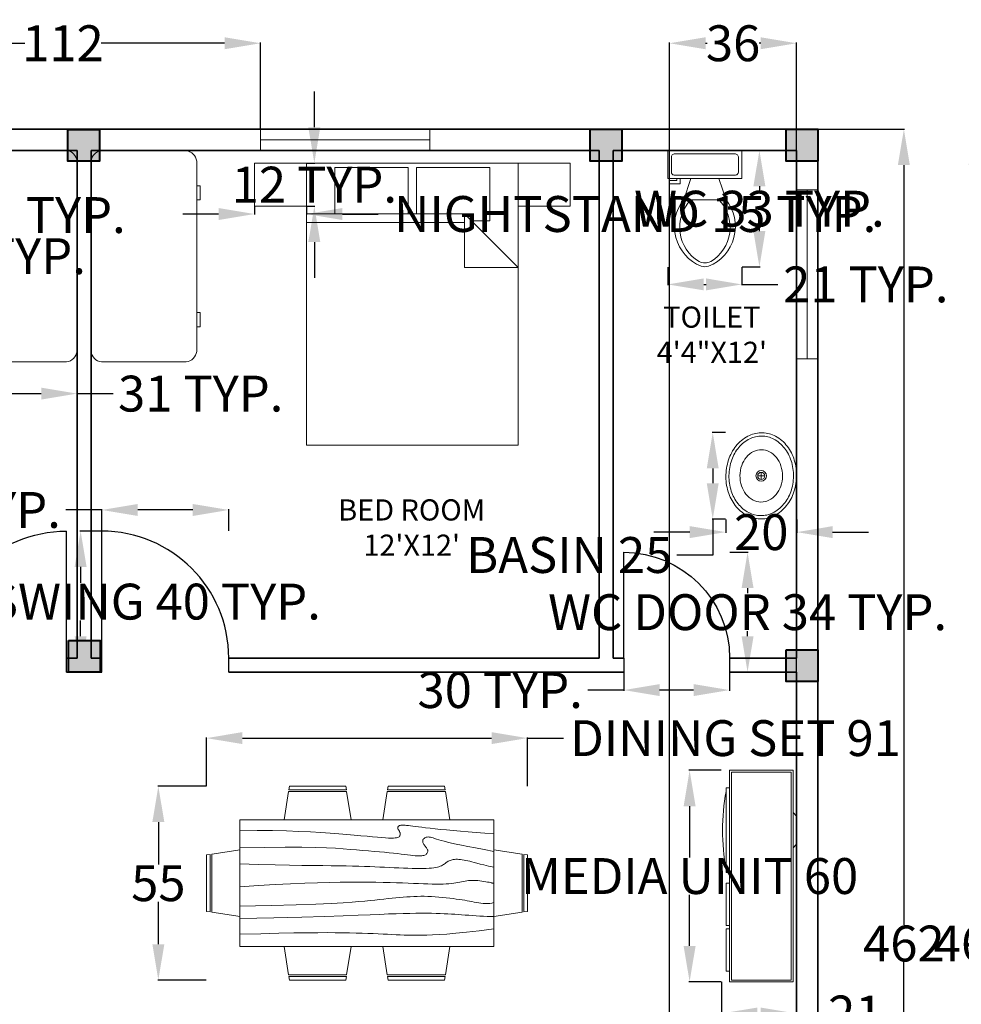
# Model space of a CAD drawing. Units: inches. Extents: x -107 to 647, y -210 to 500.
# Tile 6 of 7: x 183 to 450, y 216 to 495. Entities that reach past the tile are written whole.
import ezdxf

# ---------------------------------------------------------------- set-up
doc = ezdxf.new("R2010")
doc.units = ezdxf.units.IN
doc.header["$MEASUREMENT"] = 0
for name, color, linetype, lineweight in [('A-ANNO-DIMS', 2, 'Continuous', 18), ('A-AREA-IDEN', 7, 'Continuous', 18), ('A-COLS', 7, 'Continuous', 40), ('A-DOOR', 3, 'Continuous', 25), ('A-FLOR-FIXT', 9, 'Continuous', 18), ('A-FURN', 8, 'Continuous', 18), ('A-GLAZ', 4, 'Continuous', 18), ('A-WALL', 7, 'Continuous', 35)]:
    doc.layers.add(name, color=color, linetype=linetype, lineweight=lineweight)
doc.styles.get("Standard").update_dxf_attribs({"font": 'arial.ttf'})
doc.dimstyles.get("Standard").update_dxf_attribs({"dimtxt": 10.18, "dimasz": 10.18, "dimexe": 0.18, "dimexo": 0.0625, "dimgap": 0.09, "dimtad": 0, "dimtih": 1, "dimtoh": 1, "dimdec": 0, "dimzin": 0, "dimdsep": 46, "dimlunit": 3, "dimtxsty": 'Standard', "dimcen": 0.09, "dimadec": 0, "dimazin": 0, "dimtfac": 1, "dimtdec": 0, "dimtofl": 0, "dimtmove": 0, "dimatfit": 3, "dimfxl": 1, "dimtolj": 1, "dimtzin": 0, "dimarcsym": 0})

# ---------------------------------------------------------------- blocks, each defined once
blk = doc.blocks.new('Entertainment Center')
for p, q in [((-4, 0), (-5, -1)), ((4, 0), (-4, 0)), ((5, -1), (4, 0)), ((-17, -19), (-17, -1)), ((-17, -1), (43, -1)), ((-16.5, -18.5), (-16.5, -1.5)), ((-16.5, -1.5), (42.5, -1.5)), ((42.5, -1.5), (42.5, -18.5)), ((43, -1), (43, -19)), ((43, -19), (-17, -19)), ((42.5, -18.5), (-16.5, -18.5)), ((-12, -20), (-12, -19)), ((12, -19), (12, -20)), ((15, -20), (15, -19)), ((27, -19), (27, -20)), ((28, -20), (28, -19)), ((40, -19), (40, -20)), ((12, -20), (-12, -20)), ((27, -20), (15, -20)), ((40, -20), (28, -20))]:
    blk.add_line(p, q)
blk.add_arc((0, 40), 61, 259.6111, 280.3889)
blk = doc.blocks.new('Bed - Queen')
for p, q in [((0, -80.00003), (0, 0)), ((0, 0), (59.99999, 0)), ((59.99999, 0), (59.99999, -80.00003)), ((7.99999, -1.2), (28.79998, -1.2)), ((7.99999, -14.4), (7.99999, -1.2)), ((28.79998, -1.2), (28.79998, -14.4)), ((31.19999, -1.2), (51.99999, -1.2)), ((31.19999, -14.4), (31.19999, -1.2)), ((51.99999, -1.2), (51.99999, -16.4)), ((0, -14.4), (44.8, -14.4)), ((59.99999, -29.6), (44.8, -14.4)), ((44.8, -14.4), (44.8, -29.6)), ((51.99999, -16.4), (46.79936, -16.4)), ((44.8, -16.8), (0, -16.8)), ((44.8, -29.6), (59.99999, -29.6)), ((59.99999, -80.00003), (0, -80.00003))]:
    blk.add_line(p, q)
blk = doc.blocks.new('Desk - 30 x 60 in.')
for p, q in [((-26.999995, 0), (26.999995, 0)), ((-29.999995, -27), (-29.999995, -3)), ((29.999995, -3), (29.999995, -27)), ((26.999995, -30), (-26.999995, -30)), ((-20.000005, -30), (-20.000005, -31)), ((-16.000005, -31), (-16.000005, -30)), ((15.999995, -31), (15.999995, -30)), ((19.999995, -30), (19.999995, -31)), ((-20.000005, -31), (-16.000005, -31)), ((19.999995, -31), (15.999995, -31))]:
    blk.add_line(p, q)
for centre, start, end in [((-26.499995, -3.5), 98.1301, 171.8699), ((26.499995, -3.5), 8.130102, 81.8699), ((-26.499995, -26.5), 188.1301, 261.8699), ((26.499995, -26.5), 278.1301, 351.8699)]:
    blk.add_arc(centre, 3.535534, start, end)
blk = doc.blocks.new('Dining Set - 36 x 72 in.')
for p, q in [((-22.2343, 26.00059), (-23.4847, 17.99762)), ((-22.2304, 26), (-5.7608, 26)), ((-22, 27.5), (-22.1562, 26.50042)), ((-5.8416, 26.5), (-22.1534, 26.5)), ((-22, 27.5), (-6, 27.5)), ((-5.8437, 26.49966), (-6, 27.5)), ((-4.5152, 17.99762), (-5.7655, 25.99926)), ((5.7657, 26.00059), (4.5153, 17.99762)), ((5.7696, 26), (22.2392, 26)), ((6, 27.5), (5.8438, 26.50042)), ((22.1584, 26.5), (5.8466, 26.5)), ((6, 27.5), (22, 27.5)), ((22.1563, 26.49966), (22, 27.5)), ((23.4848, 17.99762), (22.2345, 25.99926)), ((36, 18), (-36, 18)), ((-36, 18), (-36, -18)), ((36, -18), (36, 18)), ((-44.0006, 8.23428), (-35.9976, 9.48474)), ((44.0006, 8.23428), (35.9976, 9.48474)), ((-45.5, 8), (-44.5004, 8.15617)), ((-45.5, 8), (-45.5, -8)), ((-44.5, -8.15843), (-44.5, 8.15338)), ((-44, 8.23041), (-44, -8.23915)), ((44, 8.23041), (44, -8.23915)), ((44.5, -8.15843), (44.5, 8.15338)), ((45.5, 8), (44.5005, 8.15617)), ((45.5, 8), (45.5, -8)), ((-44.4997, -8.15631), (-45.5, -8)), ((-35.9976, -9.48476), (-43.9993, -8.2345)), ((35.9976, -9.48476), (43.9993, -8.2345)), ((44.4997, -8.15631), (45.5, -8)), ((-36, -18), (36, -18)), ((-22.2343, -26.0006), (-23.4847, -17.99762)), ((-4.5152, -17.99762), (-5.7655, -25.99928)), ((5.7657, -26.0006), (4.5153, -17.99762)), ((23.4848, -17.99762), (22.2345, -25.99928)), ((-22.2304, -26), (-5.7608, -26)), ((-22, -27.5), (-22.1562, -26.50044)), ((-5.8416, -26.5), (-22.1534, -26.5)), ((-22, -27.5), (-6, -27.5)), ((-5.8437, -26.49967), (-6, -27.5)), ((5.7696, -26), (22.2392, -26)), ((6, -27.5), (5.8438, -26.50044)), ((22.1584, -26.5), (5.8466, -26.5)), ((6, -27.5), (22, -27.5)), ((22.1563, -26.49967), (22, -27.5))]:
    blk.add_line(p, q)
for points in [[(-36, 15), (-31.1772, 14.97754), (-26.8079, 14.91406), (-22.8538, 14.81543), (-19.276, 14.6875), (-16.0362, 14.53613), (-13.0957, 14.36718), (-10.4159, 14.18652), (-7.9583, 14), (-5.6904, 13.81315), (-3.6035, 13.63021), (-1.6954, 13.45508), (0.0365, 13.29166), (1.5945, 13.14388), (2.9811, 13.01562), (4.1988, 12.9108), (5.25, 12.83333), (6.1393, 12.78613), (6.8802, 12.76823), (7.4883, 12.77767), (7.9792, 12.8125), (8.3685, 12.87077), (8.6719, 12.95052), (8.9049, 13.0498), (9.0833, 13.16666), (9.2205, 13.29899), (9.3216, 13.44401), (9.3895, 13.59879), (9.4271, 13.76041), (9.4373, 13.92594), (9.4232, 14.09245), (9.3875, 14.257), (9.3333, 14.41666), (9.2638, 14.56917), (9.1836, 14.71484), (9.0975, 14.85465), (9.0104, 14.98958), (8.9272, 15.1206), (8.8529, 15.2487), (8.7922, 15.37483), (8.75, 15.5), (8.7305, 15.62467), (8.7344, 15.74739), (8.7617, 15.86621), (8.8125, 15.97916), (8.8867, 16.08431), (8.9844, 16.17968), (9.1055, 16.26334), (9.25, 16.33333), (9.4189, 16.38802), (9.6172, 16.42708), (9.8506, 16.45052), (10.125, 16.45833), (10.4463, 16.45052), (10.8203, 16.42708), (11.2529, 16.38802), (11.75, 16.33333), (12.3184, 16.26318), (12.9694, 16.17838), (13.7151, 16.07991), (14.5677, 15.96875), (15.5395, 15.84586), (16.6426, 15.71224), (17.8893, 15.56884), (19.2917, 15.41666), (20.859, 15.25667), (22.5879, 15.08984), (24.4721, 14.91715), (26.5052, 14.73958), (28.6809, 14.5581), (30.9929, 14.3737), (33.4347, 14.18733), (36, 14)], [(-36, 10), (-28.9766, 10.14274), (-23.1725, 10.20442), (-18.4241, 10.19775), (-14.5677, 10.13541), (-11.4399, 10.03011), (-8.877, 9.89453), (-6.7154, 9.74137), (-4.7917, 9.58333), (-2.9698, 9.43082), (-1.2246, 9.28515), (0.4415, 9.14534), (2.026, 9.01041), (3.5266, 8.87939), (4.9408, 8.7513), (6.266, 8.62516), (7.5, 8.5), (8.6411, 8.37549), (9.6914, 8.2539), (10.6538, 8.13818), (11.5312, 8.03125), (12.3267, 7.93603), (13.043, 7.85547), (13.6831, 7.79248), (14.25, 7.75), (14.7471, 7.7303), (15.1797, 7.73307), (15.5537, 7.75732), (15.875, 7.80208), (16.1494, 7.86637), (16.3828, 7.94922), (16.5811, 8.04964), (16.75, 8.16666), (16.8944, 8.29915), (17.0143, 8.44531), (17.1089, 8.60319), (17.1771, 8.77083), (17.218, 8.94629), (17.2305, 9.1276), (17.2137, 9.31282), (17.1667, 9.5), (17.0895, 9.6875), (16.987, 9.875), (16.8649, 10.0625), (16.7292, 10.25), (16.5856, 10.4375), (16.4401, 10.625), (16.2985, 10.8125), (16.1667, 11), (16.05, 11.18733), (15.9518, 11.3737), (15.8752, 11.5581), (15.8229, 11.73958), (15.798, 11.91715), (15.8034, 12.08984), (15.842, 12.25667), (15.9167, 12.41666), (16.0295, 12.56836), (16.1784, 12.70833), (16.3605, 12.83268), (16.5729, 12.9375), (16.8127, 13.01888), (17.0768, 13.07291), (17.3625, 13.0957), (17.6667, 13.08333), (17.9894, 13.03312), (18.3418, 12.94726), (18.7382, 12.82918), (19.1927, 12.68229), (19.7195, 12.51001), (20.3327, 12.31575), (21.0465, 12.10294), (21.875, 11.875), (22.8357, 11.63354), (23.959, 11.37304), (25.2786, 11.08618), (26.8282, 10.76562), (28.6414, 10.40405), (30.752, 9.99414), (33.1936, 9.52856), (36, 9)], [(-36, 5.5), (-30.7157, 5.3348), (-26.069, 5.20963), (-21.9946, 5.11767), (-18.4271, 5.05208), (-15.3009, 5.00602), (-12.5508, 4.97265), (-10.1112, 4.94515), (-7.9167, 4.91666), (-5.909, 4.88167), (-4.0586, 4.83984), (-2.3429, 4.79215), (-0.7396, 4.73958), (0.7739, 4.6831), (2.22, 4.6237), (3.6213, 4.56233), (5, 4.5), (6.373, 4.43782), (7.7344, 4.3776), (9.0723, 4.32129), (10.375, 4.27083), (11.6309, 4.22819), (12.8281, 4.19531), (13.9551, 4.17415), (15, 4.16666), (15.954, 4.17448), (16.819, 4.19791), (17.6001, 4.23698), (18.3021, 4.29166), (18.9299, 4.36198), (19.4883, 4.44791), (19.9823, 4.54948), (20.4167, 4.66666), (20.7969, 4.79899), (21.1302, 4.94401), (21.4245, 5.09879), (21.6875, 5.26041), (21.9271, 5.42594), (22.1511, 5.59245), (22.3672, 5.757), (22.5834, 5.91666), (22.8065, 6.06868), (23.0404, 6.21093), (23.2879, 6.34147), (23.5521, 6.45833), (23.8358, 6.55957), (24.142, 6.64323), (24.4735, 6.70735), (24.8334, 6.75), (25.2235, 6.76969), (25.642, 6.76692), (26.0858, 6.74267), (26.5521, 6.69791), (27.0379, 6.63362), (27.5404, 6.55078), (28.0565, 6.45036), (28.5834, 6.33333), (29.1242, 6.19987), (29.7071, 6.04687), (30.3661, 5.87044), (31.1354, 5.66666), (32.0493, 5.43164), (33.142, 5.16146), (34.4475, 4.85221), (36, 4.5)], [(-36, -1), (-30.7915, -0.6591), (-26.0195, -0.38216), (-21.6519, -0.16284), (-17.6563, 0.00521), (-14.0005, 0.12833), (-10.6523, 0.21289), (-7.5796, 0.26522), (-4.75, 0.29166), (-2.134, 0.29793), (0.2878, 0.28711), (2.5317, 0.26163), (4.6146, 0.22396), (6.5529, 0.17651), (8.3633, 0.12174), (10.0623, 0.06209), (11.6667, 0), (13.1899, -0.06201), (14.6341, -0.1211), (15.9982, -0.17432), (17.2813, -0.21875), (18.4823, -0.25147), (19.6003, -0.26953), (20.6343, -0.27002), (21.5834, -0.25), (22.4481, -0.20768), (23.2357, -0.14584), (23.9549, -0.06836), (24.6146, 0.02083), (25.2235, 0.11784), (25.7904, 0.21875), (26.3241, 0.31966), (26.8334, 0.41666), (27.3265, 0.50618), (27.8099, 0.58593), (28.2894, 0.65397), (28.7709, 0.70833), (29.2601, 0.74707), (29.763, 0.76823), (30.2855, 0.76985), (30.8334, 0.75), (31.4088, 0.70784), (31.9994, 0.64713), (32.589, 0.57275), (33.1615, 0.48958), (33.7008, 0.4025), (34.1908, 0.3164), (34.6153, 0.23616), (34.9584, 0.16666), (35.2099, 0.11165), (35.3848, 0.07031), (35.504, 0.04069), (35.5886, 0.02083), (35.6594, 0.00879), (35.7377, 0.0026), (35.8442, 0.00032), (36, 0)], [(-36, -6.5), (-27.1843, -6.31267), (-20.084, -6.1263), (-14.469, -5.9419), (-10.1094, -5.76042), (-6.7752, -5.58285), (-4.2363, -5.41016), (-2.2629, -5.24333), (-0.625, -5.08334), (0.8708, -4.93099), (2.2715, -4.78646), (3.5872, -4.64974), (4.8281, -4.52084), (6.0046, -4.39974), (7.127, -4.28646), (8.2053, -4.18099), (9.25, -4.08334), (10.2705, -3.99382), (11.2734, -3.91407), (12.2647, -3.84603), (13.25, -3.79167), (14.2354, -3.75293), (15.2266, -3.73177), (16.2295, -3.73015), (17.25, -3.75), (18.2912, -3.79248), (19.3451, -3.85547), (20.4009, -3.93604), (21.4479, -4.03125), (22.4754, -4.13819), (23.4727, -4.25391), (24.4289, -4.37549), (25.3334, -4.5), (26.1785, -4.62492), (26.9694, -4.74935), (27.7145, -4.87281), (28.4219, -4.99479), (29.1, -5.11483), (29.7572, -5.23242), (30.4016, -5.34709), (31.0417, -5.45834), (31.6837, -5.56437), (32.3262, -5.65821), (32.9658, -5.73153), (33.599, -5.77604), (34.2224, -5.78345), (34.8327, -5.74545), (35.4264, -5.65373), (36, -5.5)], [(-36, -10), (-26.4022, -9.81299), (-18.4675, -9.62891), (-11.9839, -9.45069), (-6.7396, -9.28125), (-2.5226, -9.12354), (0.8789, -8.98047), (3.6769, -8.85498), (6.0833, -8.75), (8.2767, -8.66765), (10.3021, -8.60677), (12.1712, -8.56543), (13.8958, -8.54167), (15.4876, -8.53353), (16.9583, -8.53907), (18.3197, -8.55632), (19.5834, -8.58334), (20.7616, -8.61841), (21.8685, -8.66081), (22.9188, -8.71004), (23.9271, -8.76563), (24.9081, -8.82707), (25.8763, -8.89388), (26.8465, -8.96558), (27.8334, -9.04167), (28.8474, -9.12118), (29.8828, -9.20117), (30.93, -9.27824), (31.9792, -9.34896), (33.0205, -9.40991), (34.0443, -9.45768), (35.0407, -9.48885), (36, -9.5)], [(-36, -14.5), (-30.0881, -14.33513), (-25.0332, -14.21224), (-20.7312, -14.12647), (-17.0781, -14.07292), (-13.97, -14.04671), (-11.3027, -14.04297), (-8.9724, -14.05681), (-6.875, -14.08334), (-4.9224, -14.11833), (-3.0905, -14.16016), (-1.3709, -14.20785), (0.2448, -14.26042), (1.7647, -14.3169), (3.1973, -14.3763), (4.5507, -14.43767), (5.8333, -14.5), (7.0554, -14.5621), (8.235, -14.62175), (9.3922, -14.67652), (10.5469, -14.72396), (11.7192, -14.76164), (12.929, -14.78711), (14.1965, -14.79794), (15.5417, -14.79167), (16.9933, -14.76424), (18.6152, -14.70508), (20.4804, -14.60197), (22.6615, -14.44271), (25.2312, -14.21509), (28.2624, -13.9069), (31.8277, -13.50594), (36, -13)]]:
    blk.add_lwpolyline(points)
blk = doc.blocks.new('Sink - Oval top')
for p, q in [((-1, 0), (1, 0)), ((0, 1), (0, -1))]:
    blk.add_line(p, q)
for points in [[(-12.23, 0.39, 0.117634), (-11.46, -3.36, 0.104469), (-8.88, -6.8, 0.090016), (-5.08, -9.07, 0.08192), (-0.32, -10.02, 0.08192), (4.49, -9.38, 0.090016), (8.42, -7.36, 0.104469), (11.22, -4.09, 0.117634), (12.23, -0.39, 0.117634), (11.46, 3.36, 0.104469), (8.88, 6.8, 0.090016), (5.08, 9.07, 0.08192), (0.32, 10.02, 0.08192), (-4.49, 9.38, 0.090016), (-8.42, 7.36, 0.104469), (-11.22, 4.09, 0.117634)], [(-11.29, 0.16, 0.118622), (-10.52, -3.25, 0.104678), (-8.07, -6.36, 0.089562), (-4.54, -8.37, 0.081185), (-0.13, -9.15, 0.081185), (4.3, -8.49, 0.089562), (7.89, -6.58, 0.104678), (10.42, -3.55, 0.118622), (11.29, -0.16, 0.118622), (10.52, 3.25, 0.104678), (8.07, 6.36, 0.089562), (4.54, 8.37, 0.081185), (0.13, 9.15, 0.081185), (-4.3, 8.49, 0.089562), (-7.89, 6.58, 0.104678), (-10.42, 3.55, 0.118622)], [(-7.42, 0.08, 0.118283), (-6.91, -2.17, 0.104607), (-5.29, -4.21, 0.089718), (-2.97, -5.53, 0.081436), (-0.07, -6.04, 0.081436), (2.84, -5.59, 0.089718), (5.2, -4.33, 0.104607), (6.86, -2.32, 0.118283), (7.42, -0.08, 0.118283), (6.91, 2.17, 0.104607), (5.29, 4.21, 0.089718), (2.97, 5.53, 0.081436), (0.07, 6.04, 0.081436), (-2.84, 5.59, 0.089718), (-5.2, 4.33, 0.104607), (-6.86, 2.32, 0.118283)]]:
    blk.add_lwpolyline(points, format="xyb", close=True)
for radius in [1.5, 1]:
    blk.add_circle((0, 0), radius)
blk = doc.blocks.new('Toilet - top')
for p, q in [((9.5, -6), (9.5, -2)), ((-8, -8.5), (-8, -8)), ((-7, -8), (-7, -9.5)), ((-4, -8), (-6, -14)), ((4, -8), (6, -14)), ((-10, -8.5), (-8, -8.5)), ((-10, -9.5), (-10, -8.5)), ((-7, -9.5), (-10, -9.5)), ((4, -14), (-4, -14))]:
    blk.add_line(p, q)
blk.add_lwpolyline([(10.5, -8), (10.5, 0), (-10.5, 0), (-10.5, -8)], close=True)
for points in [[(-9.5, -2), (-9.5, -6)], [(8.5, -1), (-8.5, -1)], [(-8.5, -7), (8.5, -7)]]:
    blk.add_lwpolyline(points)
for centre, radius, start, end in [((-8.62, -1.88), 0.884, 81.8699, 188.1301), ((8.62, -1.88), 0.884, 351.8699, 98.1301), ((-8.62, -6.12), 0.884, 171.8699, 278.1301), ((8.62, -6.12), 0.884, 261.8699, 8.1301), ((3.52, -21.58), 12.17, 141.4691, 247.9714), ((4.2, -21.82), 11.33, 136.3677, 238.9468), ((-3.52, -21.58), 12.17, 292.0284, 38.5307), ((-4.2, -21.82), 11.33, 301.053, 43.6321), ((0, -27.88), 4, 245.7318, 294.2682), ((0, -29), 4, 254.8605, 285.1395)]:
    blk.add_arc(centre, radius, start, end)
blk = doc.blocks.new('DOOR-SWING-36IN')
for p, q in [((-36, 4), (-36, 0)), ((0, 4), (0, 0)), ((0, 0), (0, -36))]:
    blk.add_line(p, q)
blk.add_arc((0, 0), 36, 180, 270)
blk = doc.blocks.new('DOOR-SWING-30IN')
for p, q in [((0, 0), (4, 0)), ((0, 0), (-30, 0)), ((0, -30), (4, -30))]:
    blk.add_line(p, q)
blk.add_arc((0, 0), 30, 180, 270)
blk = doc.blocks.new('WINDOW-48IN')
for p, q in [((0, 6), (0, 0)), ((48, 6), (48, 0)), ((0, 3), (48, 3))]:
    blk.add_line(p, q)
blk = doc.blocks.new('NIGHTSTAND-15IN')
blk.add_lwpolyline([(14.75, 12.23), (0, 12.23), (0, 0), (14.75, 0)], close=True)
blk = doc.blocks.new('COLUMN-9X9IN')
blk.add_lwpolyline([(0, 9), (9, 9), (9, 0), (0, 0)], close=True)
blk.add_solid([(0, 9), (0, 0), (9, 9), (9, 0)])
blk = doc.blocks.new('*D30')
at = {"layer": 'A-ANNO-DIMS', "color": 0, "lineweight": -2, "transparency": 16777216}
for p, q in [((206.02, 350.33), (199.9, 350.33)), ((200.08, 340.15), (200.08, 335.68)), ((200.08, 320.51), (200.08, 324.97)), ((206.02, 310.33), (199.9, 310.33))]:
    blk.add_line(p, q, dxfattribs=at)
at = {"layer": 'A-ANNO-DIMS', "color": 0, "transparency": 16777216}
for points in [[(198.39, 340.15), (201.78, 340.15), (200.08, 350.33)], [(198.39, 320.51), (201.78, 320.51), (200.08, 310.33)]]:
    blk.add_solid(points, dxfattribs=at)
at = {"layer": 'Defpoints', "color": 0, "transparency": 16777216}
for p in [(206.08, 350.33), (200.08, 310.33), (206.08, 310.33)]:
    blk.add_point(p, dxfattribs=at)
at = {"layer": 'A-ANNO-DIMS', "color": 0, "transparency": 16777216, "insert": (200.08, 330.33), "char_height": 10.18, "attachment_point": 5}
blk.add_mtext('\\A1;DOOR SWING 40 TYP.', dxfattribs=at)
blk = doc.blocks.new('*D31')
at = {"layer": 'A-ANNO-DIMS', "color": 0, "lineweight": -2, "transparency": 16777216}
for p, q in [((206.08, 356.33), (195.9, 356.33)), ((206.08, 350.39), (206.08, 356.51)), ((231.9, 356.33), (216.26, 356.33)), ((242.08, 350.39), (242.08, 356.51))]:
    blk.add_line(p, q, dxfattribs=at)
at = {"layer": 'A-ANNO-DIMS', "color": 0, "transparency": 16777216}
for points in [[(216.26, 358.02), (216.26, 354.63), (206.08, 356.33)], [(231.9, 358.02), (231.9, 354.63), (242.08, 356.33)]]:
    blk.add_solid(points, dxfattribs=at)
at = {"layer": 'Defpoints', "color": 0, "transparency": 16777216}
for p in [(206.08, 356.33), (206.08, 350.33), (242.08, 350.33)]:
    blk.add_point(p, dxfattribs=at)
at = {"layer": 'A-ANNO-DIMS', "color": 0, "transparency": 16777216, "insert": (171.04, 356.33), "char_height": 10.18, "attachment_point": 5}
blk.add_mtext('\\A1;36 TYP.', dxfattribs=at)
blk = doc.blocks.new('*D32')
at = {"layer": 'A-ANNO-DIMS', "color": 0, "lineweight": -2, "transparency": 16777216}
for p, q in [((384.14, 344.33), (389.36, 344.33)), ((389.18, 334.15), (389.18, 332.69)), ((389.18, 320.51), (389.18, 321.96)), ((384.14, 310.33), (389.36, 310.33))]:
    blk.add_line(p, q, dxfattribs=at)
at = {"layer": 'A-ANNO-DIMS', "color": 0, "transparency": 16777216}
for points in [[(387.49, 334.15), (390.88, 334.15), (389.18, 344.33)], [(387.49, 320.51), (390.88, 320.51), (389.18, 310.33)]]:
    blk.add_solid(points, dxfattribs=at)
at = {"layer": 'Defpoints', "color": 0, "transparency": 16777216}
for p in [(384.08, 344.33), (384.08, 310.33), (389.18, 310.33)]:
    blk.add_point(p, dxfattribs=at)
at = {"layer": 'A-ANNO-DIMS', "color": 0, "transparency": 16777216, "insert": (389.18, 327.33), "char_height": 10.18, "attachment_point": 5}
blk.add_mtext('\\A1;WC DOOR 34 TYP.', dxfattribs=at)
blk = doc.blocks.new('*D33')
at = {"layer": 'A-ANNO-DIMS', "color": 0, "lineweight": -2, "transparency": 16777216}
for p, q in [((354.08, 310.26), (354.08, 305.05)), ((384.08, 310.26), (384.08, 305.05)), ((354.08, 305.23), (343.9, 305.23)), ((373.9, 305.23), (364.26, 305.23))]:
    blk.add_line(p, q, dxfattribs=at)
at = {"layer": 'A-ANNO-DIMS', "color": 0, "transparency": 16777216}
for points in [[(364.26, 306.92), (364.26, 303.53), (354.08, 305.23)], [(373.9, 306.92), (373.9, 303.53), (384.08, 305.23)]]:
    blk.add_solid(points, dxfattribs=at)
at = {"layer": 'Defpoints', "color": 0, "transparency": 16777216}
for p in [(354.08, 310.33), (384.08, 310.33), (354.08, 305.23)]:
    blk.add_point(p, dxfattribs=at)
at = {"layer": 'A-ANNO-DIMS', "color": 0, "transparency": 16777216, "insert": (319.04, 305.23), "char_height": 10.18, "attachment_point": 5}
blk.add_mtext('\\A1;30 TYP.', dxfattribs=at)
blk = doc.blocks.new('*D38')
at = {"layer": 'A-ANNO-DIMS', "color": 0, "lineweight": -2, "transparency": 16777216}
for p, q in [((382.93, 378.28), (379.13, 378.28)), ((379.31, 368.1), (379.31, 363.91)), ((382.93, 353.73), (379.13, 353.73)), ((379.31, 353.73), (379.31, 343.55)), ((379.31, 343.55), (369.13, 343.55))]:
    blk.add_line(p, q, dxfattribs=at)
at = {"layer": 'A-ANNO-DIMS', "color": 0, "transparency": 16777216}
for points in [[(377.61, 368.1), (381, 368.1), (379.31, 378.28)], [(377.61, 363.91), (381, 363.91), (379.31, 353.73)]]:
    blk.add_solid(points, dxfattribs=at)
at = {"layer": 'Defpoints', "color": 0, "transparency": 16777216}
for p in [(382.99, 378.28), (379.31, 353.73), (382.99, 353.73)]:
    blk.add_point(p, dxfattribs=at)
at = {"layer": 'A-ANNO-DIMS', "color": 0, "transparency": 16777216, "insert": (338.62, 343.55), "char_height": 10.18, "attachment_point": 5}
blk.add_mtext('\\A1;BASIN 25', dxfattribs=at)
blk = doc.blocks.new('*D39')
at = {"layer": 'A-ANNO-DIMS', "color": 0, "lineweight": -2, "transparency": 16777216}
for p, q in [((382.99, 353.66), (382.99, 349.86)), ((403.13, 353.66), (403.13, 349.86)), ((372.81, 350.04), (362.63, 350.04)), ((413.31, 350.04), (423.49, 350.04))]:
    blk.add_line(p, q, dxfattribs=at)
at = {"layer": 'A-ANNO-DIMS', "color": 0, "transparency": 16777216}
for points in [[(372.81, 351.74), (372.81, 348.35), (382.99, 350.04)], [(413.31, 351.74), (413.31, 348.35), (403.13, 350.04)]]:
    blk.add_solid(points, dxfattribs=at)
at = {"layer": 'Defpoints', "color": 0, "transparency": 16777216}
for p in [(382.99, 353.73), (403.13, 353.73), (403.13, 350.04)]:
    blk.add_point(p, dxfattribs=at)
at = {"layer": 'A-ANNO-DIMS', "color": 0, "transparency": 16777216, "insert": (393.06, 350.04), "char_height": 10.18, "attachment_point": 5}
blk.add_mtext('\\A1;20', dxfattribs=at)
blk = doc.blocks.new('*D44')
at = {"layer": 'A-ANNO-DIMS', "color": 0, "lineweight": -2, "transparency": 16777216}
for p, q in [((168.03, 458.34), (158.91, 458.34)), ((159.09, 448.16), (159.09, 433.69)), ((159.09, 408.52), (159.09, 422.98)), ((168.03, 398.34), (158.91, 398.34))]:
    blk.add_line(p, q, dxfattribs=at)
at = {"layer": 'A-ANNO-DIMS', "color": 0, "transparency": 16777216}
for points in [[(157.39, 448.16), (160.78, 448.16), (159.09, 458.34)], [(157.39, 408.52), (160.78, 408.52), (159.09, 398.34)]]:
    blk.add_solid(points, dxfattribs=at)
at = {"layer": 'Defpoints', "color": 0, "transparency": 16777216}
for p in [(168.09, 458.34), (159.09, 398.34), (168.09, 398.34)]:
    blk.add_point(p, dxfattribs=at)
at = {"layer": 'A-ANNO-DIMS', "color": 0, "transparency": 16777216, "insert": (159.09, 428.34), "char_height": 10.18, "attachment_point": 5}
blk.add_mtext('\\A1;DESK 60 TYP.', dxfattribs=at)
blk = doc.blocks.new('*D45')
at = {"layer": 'A-ANNO-DIMS', "color": 0, "lineweight": -2, "transparency": 16777216}
for p, q in [((168.09, 398.27), (168.09, 389.16)), ((199.09, 398.27), (199.09, 389.16)), ((178.27, 389.34), (188.91, 389.34)), ((199.09, 389.34), (209.27, 389.34))]:
    blk.add_line(p, q, dxfattribs=at)
at = {"layer": 'A-ANNO-DIMS', "color": 0, "transparency": 16777216}
for points in [[(178.27, 391.03), (178.27, 387.64), (168.09, 389.34)], [(188.91, 391.03), (188.91, 387.64), (199.09, 389.34)]]:
    blk.add_solid(points, dxfattribs=at)
at = {"layer": 'Defpoints', "color": 0, "transparency": 16777216}
for p in [(168.09, 398.34), (199.09, 398.34), (199.09, 389.34)]:
    blk.add_point(p, dxfattribs=at)
at = {"layer": 'A-ANNO-DIMS', "color": 0, "transparency": 16777216, "insert": (234.13, 389.34), "char_height": 10.18, "attachment_point": 5}
blk.add_mtext('\\A1;31 TYP.', dxfattribs=at)
blk = doc.blocks.new('*D46')
at = {"layer": 'A-ANNO-DIMS', "color": 0, "lineweight": -2, "transparency": 16777216}
for p, q in [((387.64, 458.33), (392.72, 458.33)), ((392.54, 448.15), (392.54, 447.16)), ((392.54, 435.46), (392.54, 436.44)), ((387.64, 425.28), (392.72, 425.28))]:
    blk.add_line(p, q, dxfattribs=at)
at = {"layer": 'A-ANNO-DIMS', "color": 0, "transparency": 16777216}
for points in [[(390.84, 448.15), (394.24, 448.15), (392.54, 458.33)], [(390.84, 435.46), (394.24, 435.46), (392.54, 425.28)]]:
    blk.add_solid(points, dxfattribs=at)
at = {"layer": 'Defpoints', "color": 0, "transparency": 16777216}
for p in [(387.58, 458.33), (392.54, 458.33), (387.58, 425.28)]:
    blk.add_point(p, dxfattribs=at)
at = {"layer": 'A-ANNO-DIMS', "color": 0, "transparency": 16777216, "insert": (392.54, 441.8), "char_height": 10.18, "attachment_point": 5}
blk.add_mtext('\\A1;WC 33 TYP.', dxfattribs=at)
blk = doc.blocks.new('*D47')
at = {"layer": 'A-ANNO-DIMS', "color": 0, "lineweight": -2, "transparency": 16777216}
for p, q in [((366.58, 425.22), (366.58, 420.14)), ((387.58, 425.22), (387.58, 420.14)), ((376.76, 420.32), (377.4, 420.32)), ((387.58, 420.32), (397.76, 420.32))]:
    blk.add_line(p, q, dxfattribs=at)
at = {"layer": 'A-ANNO-DIMS', "color": 0, "transparency": 16777216}
for points in [[(376.76, 422.02), (376.76, 418.63), (366.58, 420.32)], [(377.4, 422.02), (377.4, 418.63), (387.58, 420.32)]]:
    blk.add_solid(points, dxfattribs=at)
at = {"layer": 'Defpoints', "color": 0, "transparency": 16777216}
for p in [(366.58, 425.28), (387.58, 425.28), (387.58, 420.32)]:
    blk.add_point(p, dxfattribs=at)
at = {"layer": 'A-ANNO-DIMS', "color": 0, "transparency": 16777216, "insert": (422.71, 420.32), "char_height": 10.18, "attachment_point": 5}
blk.add_mtext('\\A1;21 TYP.', dxfattribs=at)
blk = doc.blocks.new('*D50')
at = {"layer": 'A-ANNO-DIMS', "color": 0, "lineweight": -2, "transparency": 16777216}
for p, q in [((38.19, 441.9), (38.19, 439.81)), ((51.33, 441.9), (51.33, 439.81)), ((28.01, 439.99), (17.83, 439.99)), ((61.51, 439.99), (71.69, 439.99))]:
    blk.add_line(p, q, dxfattribs=at)
at = {"layer": 'A-ANNO-DIMS', "color": 0, "transparency": 16777216}
for points in [[(28.01, 441.69), (28.01, 438.29), (38.19, 439.99)], [(61.51, 441.69), (61.51, 438.29), (51.33, 439.99)]]:
    blk.add_solid(points, dxfattribs=at)
at = {"layer": 'Defpoints', "color": 0, "transparency": 16777216}
for p in [(38.19, 441.96), (51.33, 441.96), (51.33, 439.99)]:
    blk.add_point(p, dxfattribs=at)
at = {"layer": 'A-ANNO-DIMS', "color": 0, "transparency": 16777216, "insert": (144.5, 439.99), "char_height": 10.18, "attachment_point": 5}
blk.add_mtext('\\A1;NIGHTSTAND 13 TYP.', dxfattribs=at)
blk = doc.blocks.new('*D52')
at = {"layer": 'A-ANNO-DIMS', "color": 0, "lineweight": -2, "transparency": 16777216}
for p, q in [((249.38, 442.44), (249.38, 440.11)), ((264.13, 442.44), (264.13, 440.11)), ((239.2, 440.29), (229.02, 440.29)), ((274.31, 440.29), (284.49, 440.29))]:
    blk.add_line(p, q, dxfattribs=at)
at = {"layer": 'A-ANNO-DIMS', "color": 0, "transparency": 16777216}
for points in [[(239.2, 441.99), (239.2, 438.59), (249.38, 440.29)], [(274.31, 441.99), (274.31, 438.59), (264.13, 440.29)]]:
    blk.add_solid(points, dxfattribs=at)
at = {"layer": 'Defpoints', "color": 0, "transparency": 16777216}
for p in [(249.38, 442.5), (264.13, 442.5), (264.13, 440.29)]:
    blk.add_point(p, dxfattribs=at)
at = {"layer": 'A-ANNO-DIMS', "color": 0, "transparency": 16777216, "insert": (357.31, 440.29), "char_height": 10.18, "attachment_point": 5}
blk.add_mtext('\\A1;NIGHTSTAND 15 TYP.', dxfattribs=at)
blk = doc.blocks.new('*D53')
at = {"layer": 'A-ANNO-DIMS', "color": 0, "lineweight": -2, "transparency": 16777216}
for p, q in [((266.35, 464.91), (266.35, 475.09)), ((264.2, 454.73), (266.53, 454.73)), ((264.2, 442.5), (266.53, 442.5)), ((266.35, 432.32), (266.35, 422.14))]:
    blk.add_line(p, q, dxfattribs=at)
at = {"layer": 'A-ANNO-DIMS', "color": 0, "transparency": 16777216}
for points in [[(264.65, 464.91), (268.04, 464.91), (266.35, 454.73)], [(264.65, 432.32), (268.04, 432.32), (266.35, 442.5)]]:
    blk.add_solid(points, dxfattribs=at)
at = {"layer": 'Defpoints', "color": 0, "transparency": 16777216}
for p in [(264.13, 454.73), (266.35, 454.73), (264.13, 442.5)]:
    blk.add_point(p, dxfattribs=at)
at = {"layer": 'A-ANNO-DIMS', "color": 0, "transparency": 16777216, "insert": (266.35, 448.62), "char_height": 10.18, "attachment_point": 5}
blk.add_mtext('\\A1;12 TYP.', dxfattribs=at)
blk = doc.blocks.new('*D58')
at = {"layer": 'A-ANNO-DIMS', "color": 0, "lineweight": -2, "transparency": 16777216}
for p, q in [((381.69, 282.47), (372.57, 282.47)), ((372.75, 272.29), (372.75, 257.76)), ((372.75, 232.65), (372.75, 247.18)), ((381.69, 222.47), (372.57, 222.47))]:
    blk.add_line(p, q, dxfattribs=at)
at = {"layer": 'A-ANNO-DIMS', "color": 0, "transparency": 16777216}
for points in [[(371.05, 272.29), (374.45, 272.29), (372.75, 282.47)], [(371.05, 232.65), (374.45, 232.65), (372.75, 222.47)]]:
    blk.add_solid(points, dxfattribs=at)
at = {"layer": 'Defpoints', "color": 0, "transparency": 16777216}
for p in [(381.75, 282.47), (372.75, 222.47), (381.75, 222.47)]:
    blk.add_point(p, dxfattribs=at)
at = {"layer": 'A-ANNO-DIMS', "color": 0, "transparency": 16777216, "insert": (372.75, 252.47), "char_height": 10.18, "attachment_point": 5}
blk.add_mtext('\\A1;MEDIA UNIT 60', dxfattribs=at)
blk = doc.blocks.new('*D59')
at = {"layer": 'A-ANNO-DIMS', "color": 0, "lineweight": -2, "transparency": 16777216}
for p, q in [((381.75, 222.41), (381.75, 213.29)), ((403.08, 222.41), (403.08, 213.29)), ((391.93, 213.47), (392.9, 213.47)), ((403.08, 213.47), (413.26, 213.47))]:
    blk.add_line(p, q, dxfattribs=at)
at = {"layer": 'A-ANNO-DIMS', "color": 0, "transparency": 16777216}
for points in [[(391.93, 215.16), (391.93, 211.77), (381.75, 213.47)], [(392.9, 215.16), (392.9, 211.77), (403.08, 213.47)]]:
    blk.add_solid(points, dxfattribs=at)
at = {"layer": 'Defpoints', "color": 0, "transparency": 16777216}
for p in [(381.75, 222.47), (403.08, 222.47), (403.08, 213.47)]:
    blk.add_point(p, dxfattribs=at)
at = {"layer": 'A-ANNO-DIMS', "color": 0, "transparency": 16777216, "insert": (419.75, 213.47), "char_height": 10.18, "attachment_point": 5}
blk.add_mtext('\\A1;21', dxfattribs=at)
blk = doc.blocks.new('*D66')
at = {"layer": 'A-ANNO-DIMS', "color": 0, "lineweight": -2, "transparency": 16777216}
for p, q in [((235.77, 278.01), (235.77, 291.78)), ((245.95, 291.6), (316.59, 291.6)), ((326.77, 278.01), (326.77, 291.78)), ((326.77, 291.6), (336.95, 291.6))]:
    blk.add_line(p, q, dxfattribs=at)
at = {"layer": 'A-ANNO-DIMS', "color": 0, "transparency": 16777216}
for points in [[(245.95, 293.3), (245.95, 289.91), (235.77, 291.6)], [(316.59, 293.3), (316.59, 289.91), (326.77, 291.6)]]:
    blk.add_solid(points, dxfattribs=at)
at = {"layer": 'Defpoints', "color": 0, "transparency": 16777216}
for p in [(326.77, 291.6), (235.77, 277.95), (326.77, 277.95)]:
    blk.add_point(p, dxfattribs=at)
at = {"layer": 'A-ANNO-DIMS', "color": 0, "transparency": 16777216, "insert": (385.76, 291.6), "char_height": 10.18, "attachment_point": 5}
blk.add_mtext('\\A1;DINING SET 91', dxfattribs=at)
blk = doc.blocks.new('*D67')
at = {"layer": 'A-ANNO-DIMS', "color": 0, "lineweight": -2, "transparency": 16777216}
for p, q in [((235.71, 277.95), (221.94, 277.95)), ((222.12, 267.77), (222.12, 255.72)), ((222.12, 233.13), (222.12, 245.19)), ((235.71, 222.95), (221.94, 222.95))]:
    blk.add_line(p, q, dxfattribs=at)
at = {"layer": 'A-ANNO-DIMS', "color": 0, "transparency": 16777216}
for points in [[(220.42, 267.77), (223.82, 267.77), (222.12, 277.95)], [(220.42, 233.13), (223.82, 233.13), (222.12, 222.95)]]:
    blk.add_solid(points, dxfattribs=at)
at = {"layer": 'Defpoints', "color": 0, "transparency": 16777216}
for p in [(222.12, 277.95), (235.77, 277.95), (235.77, 222.95)]:
    blk.add_point(p, dxfattribs=at)
at = {"layer": 'A-ANNO-DIMS', "color": 0, "transparency": 16777216, "insert": (222.12, 250.45), "char_height": 10.18, "attachment_point": 5}
blk.add_mtext('\\A1;55', dxfattribs=at)
blk = doc.blocks.new('*D73')
at = {"layer": 'A-ANNO-DIMS', "color": 0, "lineweight": -2, "transparency": 16777216}
for p, q in [((409.14, 464.33), (433.68, 464.33)), ((433.5, 454.15), (433.5, 238.61)), ((433.5, 12.51), (433.5, 228.04)), ((409.14, 2.33), (433.68, 2.33))]:
    blk.add_line(p, q, dxfattribs=at)
at = {"layer": 'A-ANNO-DIMS', "color": 0, "transparency": 16777216}
for points in [[(431.8, 454.15), (435.19, 454.15), (433.5, 464.33)], [(431.8, 12.51), (435.19, 12.51), (433.5, 2.33)]]:
    blk.add_solid(points, dxfattribs=at)
at = {"layer": 'Defpoints', "color": 0, "transparency": 16777216}
for p in [(409.08, 464.33), (433.5, 464.33), (409.08, 2.33)]:
    blk.add_point(p, dxfattribs=at)
at = {"layer": 'A-ANNO-DIMS', "color": 0, "transparency": 16777216, "insert": (433.5, 233.33), "char_height": 10.18, "attachment_point": 5}
blk.add_mtext('\\A1;462', dxfattribs=at)
blk = doc.blocks.new('*D76')
at = {"layer": 'A-ANNO-DIMS', "color": 0, "lineweight": -2, "transparency": 16777216}
for p, q in [((139.08, 464.39), (139.08, 488.92)), ((251.08, 464.39), (251.08, 488.92)), ((149.26, 488.74), (184.28, 488.74)), ((240.9, 488.74), (205.89, 488.74))]:
    blk.add_line(p, q, dxfattribs=at)
at = {"layer": 'A-ANNO-DIMS', "color": 0, "transparency": 16777216}
for points in [[(149.26, 490.44), (149.26, 487.04), (139.08, 488.74)], [(240.9, 490.44), (240.9, 487.04), (251.08, 488.74)]]:
    blk.add_solid(points, dxfattribs=at)
at = {"layer": 'Defpoints', "color": 0, "transparency": 16777216}
for p in [(251.08, 488.74), (139.08, 464.33), (251.08, 464.33)]:
    blk.add_point(p, dxfattribs=at)
at = {"layer": 'A-ANNO-DIMS', "color": 0, "transparency": 16777216, "insert": (195.08, 488.74), "char_height": 10.18, "attachment_point": 5}
blk.add_mtext('\\A1;112', dxfattribs=at)
blk = doc.blocks.new('*D81')
at = {"layer": 'A-ANNO-DIMS', "color": 0, "lineweight": -2, "transparency": 16777216}
for p, q in [((367.08, 44.39), (367.08, 488.92)), ((403.08, 44.39), (403.08, 488.92)), ((377.26, 488.74), (377.71, 488.74)), ((392.9, 488.74), (392.46, 488.74))]:
    blk.add_line(p, q, dxfattribs=at)
at = {"layer": 'A-ANNO-DIMS', "color": 0, "transparency": 16777216}
for points in [[(377.26, 490.44), (377.26, 487.04), (367.08, 488.74)], [(392.9, 490.44), (392.9, 487.04), (403.08, 488.74)]]:
    blk.add_solid(points, dxfattribs=at)
at = {"layer": 'Defpoints', "color": 0, "transparency": 16777216}
for p in [(403.08, 488.74), (367.08, 44.33), (403.08, 44.33)]:
    blk.add_point(p, dxfattribs=at)
at = {"layer": 'A-ANNO-DIMS', "color": 0, "transparency": 16777216, "insert": (385.08, 488.74), "char_height": 10.18, "attachment_point": 5}
blk.add_mtext('\\A1;36', dxfattribs=at)
blk = doc.blocks.new('*D98')
at = {"layer": 'A-ANNO-DIMS', "color": 0, "lineweight": -2, "transparency": 16777216}
for p, q in [((476.69, 464.33), (453.37, 464.33)), ((453.55, 454.15), (453.55, 238.61)), ((453.55, 12.51), (453.55, 228.04)), ((476.69, 2.33), (453.37, 2.33))]:
    blk.add_line(p, q, dxfattribs=at)
at = {"layer": 'A-ANNO-DIMS', "color": 0, "transparency": 16777216}
for points in [[(451.85, 454.15), (455.25, 454.15), (453.55, 464.33)], [(451.85, 12.51), (455.25, 12.51), (453.55, 2.33)]]:
    blk.add_solid(points, dxfattribs=at)
at = {"layer": 'Defpoints', "color": 0, "transparency": 16777216}
for p in [(453.55, 464.33), (476.75, 464.33), (476.75, 2.33)]:
    blk.add_point(p, dxfattribs=at)
at = {"layer": 'A-ANNO-DIMS', "color": 0, "transparency": 16777216, "insert": (453.55, 233.33), "char_height": 10.18, "attachment_point": 5}
blk.add_mtext('\\A1;462', dxfattribs=at)

msp = doc.modelspace()

# ---------------------------------------------------------------- linework, layer by layer
at = {"layer": 'A-WALL'}
for p, q in [((199.082, 458.325), (31.082, 458.325)), ((199.082, 458.325), (199.082, 314.325)), ((203.082, 458.325), (203.082, 314.325)), ((347.082, 458.325), (203.082, 458.325)), ((347.082, 458.325), (347.082, 314.325)), ((403.082, 458.325), (351.082, 458.325)), ((351.082, 458.325), (351.082, 314.325)), ((403.082, 314.325), (403.082, 458.325)), ((199.082, 314.325), (196.082, 314.325)), ((206.082, 314.325), (203.082, 314.325)), ((347.082, 314.325), (242.082, 314.325)), ((354.082, 314.325), (351.082, 314.325)), ((403.082, 314.325), (384.082, 314.325)), ((206.082, 310.325), (196.082, 310.325)), ((354.082, 310.325), (242.082, 310.325)), ((403.082, 310.325), (384.082, 310.325)), ((403.082, 124.325), (403.082, 310.325))]:
    msp.add_line(p, q, dxfattribs=at)
msp.add_lwpolyline([(25.082, 2.325), (409.082, 2.325), (409.082, 464.325), (25.082, 464.325)], close=True, dxfattribs=at)

# ---------------------------------------------------------------- block references
at = {"layer": 'A-COLS'}
for p in [(196.48, 455.307), (344.561, 455.325), (400.082, 455.325), (196.602, 310.325), (400.082, 307.633)]:
    msp.add_blockref('COLUMN-9X9IN', p, dxfattribs=at)
at = {"layer": 'A-DOOR', "extrusion": (0, 0, -1), "zscale": -1}
for name, p, rotation in [('DOOR-SWING-36IN', (-196.082, 314.325), 180), ('DOOR-SWING-30IN', (-354.082, 314.325), 270)]:
    msp.add_blockref(name, p, dxfattribs=dict(at, rotation=rotation))
at = {"layer": 'A-DOOR', "rotation": 180}
msp.add_blockref('DOOR-SWING-36IN', (206.082, 314.325), dxfattribs=at)
at = {"layer": 'A-FLOR-FIXT'}
msp.add_blockref('Toilet - top', (377.082, 458.325), dxfattribs=at)
at = {"layer": 'A-FLOR-FIXT', "rotation": 270}
msp.add_blockref('Sink - Oval top', (393.058, 366.003), dxfattribs=at)
at = {"layer": 'A-FURN'}
for name, p, rotation in [('Desk - 30 x 60 in.', (199.088, 428.336), 270), ('Desk - 30 x 60 in.', (203, 428.317), 90), ('Entertainment Center', (403.082, 265.468), 270)]:
    msp.add_blockref(name, p, dxfattribs=dict(at, rotation=rotation))
for name, p in [('NIGHTSTAND-15IN', (249.38, 442.501)), ('Bed - Queen', (264.134, 454.73)), ('Dining Set - 36 x 72 in.', (281.272, 250.452))]:
    msp.add_blockref(name, p, dxfattribs=at)
at = {"layer": 'A-FURN', "extrusion": (0, 0, -1), "zscale": -1}
msp.add_blockref('NIGHTSTAND-15IN', (-338.887, 442.501), dxfattribs=at)
at = {"layer": 'A-GLAZ'}
msp.add_blockref('WINDOW-48IN', (251.082, 458.325), dxfattribs=at)
at = {"layer": 'A-GLAZ', "rotation": 269.9999999999998}
msp.add_blockref('WINDOW-48IN', (403.082, 447.198), dxfattribs=at)

# ---------------------------------------------------------------- texts
at = {"layer": 'A-AREA-IDEN', "char_height": 6, "attachment_point": 1}
for s, insert in [('\\pxqc;TOILET\\P4\'4"X12\'', (356.108, 414.049)), ("\\pxqc;BED ROOM\\P12'X12'", (271.013, 359.338))]:
    msp.add_mtext_dynamic_manual_height_columns(s, width=45.88849, gutter_width=1, heights=[0], dxfattribs=dict(at, insert=insert))

# ---------------------------------------------------------------- dimensions: what is measured, and where the dimension line sits
at = {"layer": 'A-ANNO-DIMS'}
for base, p1, p2, picture, middle in [((251.082, 488.742), (139.082, 464.325), (251.082, 464.325), '*D76', (195.082, 488.742)), ((403.082, 488.742), (367.082, 44.325), (403.082, 44.325), '*D81', (385.082, 488.742)), ((403.126, 350.045), (382.99, 353.727), (403.126, 353.727), '*D39', (393.058, 350.045)), ((403.082, 213.468), (381.748, 222.468), (403.082, 222.468), '*D59', (419.747, 213.468))]:
    dim = msp.add_linear_dim(base=base, p1=p1, p2=p2, dimstyle='Standard', override={"dimdec": 0, "dimlfac": 1, "dimrnd": 0, "dimzin": 0, "dimdsep": 46, "dimlunit": 2}, dxfattribs=at)
    dim.commit()
    dim.dimension.update_dxf_attribs({"geometry": picture, "text_midpoint": middle})
for base, p1, p2, angle, text, picture, middle in [((266.347, 454.73), (264.134, 442.501), (264.134, 454.73), 90, '<> TYP.', '*D53', (266.347, 448.615)), ((392.539, 458.325), (387.582, 425.279), (387.582, 458.325), 90, 'WC <> TYP.', '*D46', (392.539, 441.802)), ((159.088, 398.336), (168.088, 458.336), (168.088, 398.336), 270, 'DESK <> TYP.', '*D44', (159.088, 428.336)), ((379.307, 353.727), (382.99, 378.278), (382.99, 353.727), 270, 'BASIN <>', '*D38', (338.619, 343.547)), ((206.082, 356.325), (242.082, 350.325), (206.082, 350.325), 180, '<> TYP.', '*D31', (171.039, 356.325)), ((200.082, 310.325), (206.082, 350.325), (206.082, 310.325), 270, 'DOOR SWING <> TYP.', '*D30', (200.082, 330.325)), ((389.182, 310.325), (384.082, 344.325), (384.082, 310.325), 270, 'WC DOOR <> TYP.', '*D32', (389.182, 327.325)), ((354.082, 305.225), (384.082, 310.325), (354.082, 310.325), 180, '<> TYP.', '*D33', (319.039, 305.225)), ((372.748, 222.468), (381.748, 282.468), (381.748, 222.468), 270, 'MEDIA UNIT <>', '*D58', (372.748, 252.468))]:
    dim = msp.add_linear_dim(base=base, p1=p1, p2=p2, angle=angle, text=text, dimstyle='Standard', override={"dimdec": 0, "dimlfac": 1, "dimrnd": 0, "dimzin": 0, "dimdsep": 46, "dimlunit": 2}, dxfattribs=at)
    dim.commit()
    dim.dimension.update_dxf_attribs({"geometry": picture, "text_midpoint": middle})
for base, p1, p2, text, picture, middle in [((264.134, 440.288), (249.38, 442.501), (264.134, 442.501), 'NIGHTSTAND <> TYP.', '*D52', (357.309, 440.288)), ((51.328, 439.989), (38.19, 441.959), (51.328, 441.959), 'NIGHTSTAND <> TYP.', '*D50', (144.503, 439.989)), ((387.582, 420.322), (366.582, 425.279), (387.582, 425.279), '<> TYP.', '*D47', (422.715, 420.322)), ((199.088, 389.336), (168.088, 398.336), (199.088, 398.336), '<> TYP.', '*D45', (234.131, 389.336)), ((326.772, 291.602), (235.772, 277.952), (326.772, 277.952), 'DINING SET <>', '*D66', (385.765, 291.602))]:
    dim = msp.add_linear_dim(base=base, p1=p1, p2=p2, text=text, dimstyle='Standard', override={"dimdec": 0, "dimlfac": 1, "dimrnd": 0, "dimzin": 0, "dimdsep": 46, "dimlunit": 2}, dxfattribs=at)
    dim.commit()
    dim.dimension.update_dxf_attribs({"geometry": picture, "text_midpoint": middle})
for base, p1, p2, picture, middle in [((433.498, 464.325), (409.082, 2.325), (409.082, 464.325), '*D73', (433.498, 233.325)), ((453.549, 464.325), (476.749, 2.325), (476.749, 464.325), '*D98', (453.549, 233.325)), ((222.122, 277.952), (235.772, 222.952), (235.772, 277.952), '*D67', (222.122, 250.452))]:
    dim = msp.add_linear_dim(base=base, p1=p1, p2=p2, angle=90, dimstyle='Standard', override={"dimdec": 0, "dimlfac": 1, "dimrnd": 0, "dimzin": 0, "dimdsep": 46, "dimlunit": 2}, dxfattribs=at)
    dim.commit()
    dim.dimension.update_dxf_attribs({"geometry": picture, "text_midpoint": middle})

doc.saveas('drawing.dxf')
